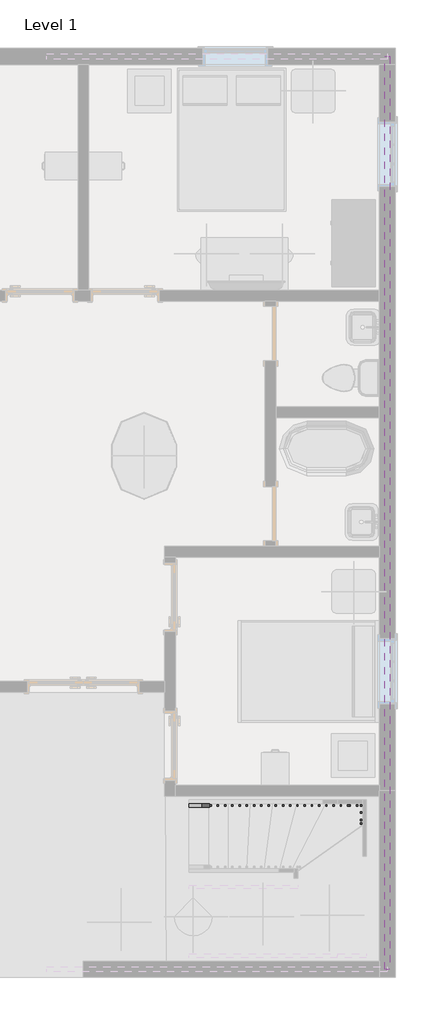
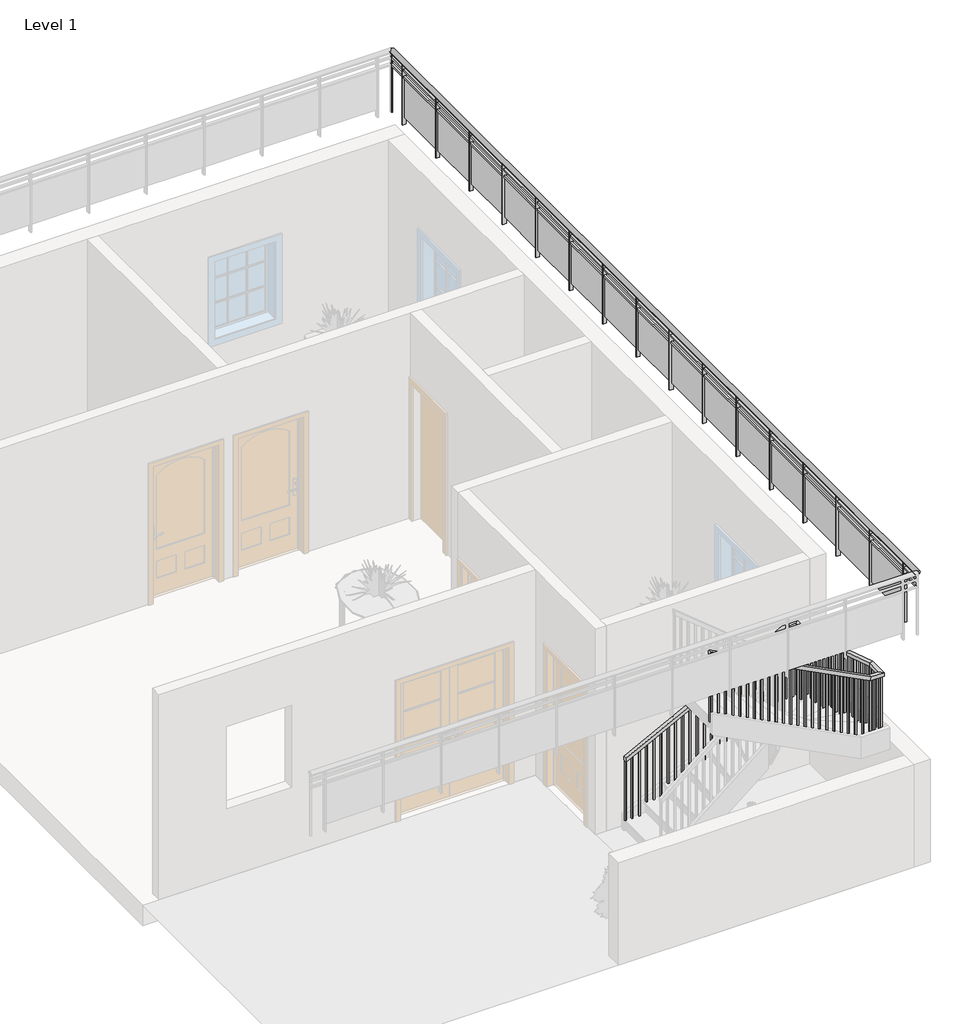
# One storey, part 3 of 4: 2 railings.
"""IFC4 building model written with IfcOpenShell, lengths in millimetres."""

from ifc_helpers import new_model, si_unit, point, frame, origin, place, context, project, spatial, polyline, ellipse_curve, trimmed, outline, extrude, faceted_brep, element, save
from ifc_brep_helpers import plane_surface, extruded_surface, advanced_brep

model = new_model("IFC4")

# Units and contexts
model_context = context("Model", 3, world=origin())
ifc_project = project(units=[si_unit("LENGTHUNIT", "METRE", prefix="MILLI")], contexts=[model_context])

# Site, building, storey
site = spatial("IfcSite", under=ifc_project)
building = spatial("IfcBuilding", under=site)
storey = spatial("IfcBuildingStorey", under=building, Name="Level 1", Elevation=0.0)

# Railings
placement = place(None, origin())
element("IfcRailing", 1, ObjectType="Glass Panel - Bottom Fill", at=placement, inside=storey, context=model_context, shape_type="SolidModel", body=[
    advanced_brep(
    [(-4161.4505662, 13087.2645941, 4267.2), (-4237.6505662, 13087.2645941, 4267.2), (-4161.4505662, 285.6645941, 4267.2), (-4237.6505662, 285.6645941, 4267.2)],
    [
        (0, 1, ellipse_curve(frame((-4199.5505662, 13087.2645941, 4267.2), z_axis=(0.0, 1.0, 0.0), x_axis=(-1.0, 0.0, 0.0)), 38.1, 28.575)),
        (1, 0, ellipse_curve(frame((-4199.5505662, 13087.2645941, 4267.2), z_axis=(0.0, 1.0, 0.0), x_axis=(-1.0, 0.0, 0.0)), 38.1, 28.575)),
        (2, 3, ellipse_curve(frame((-4199.5505662, 285.6645941, 4267.2), z_axis=(0.0, -1.0, 0.0), x_axis=(-1.0, 0.0, 0.0)), 38.1, 28.575)),
        (3, 2, ellipse_curve(frame((-4199.5505662, 285.6645941, 4267.2), z_axis=(0.0, -1.0, 0.0), x_axis=(-1.0, 0.0, 0.0)), 38.1, 28.575)),
        (0, 2),
        (3, 1),
    ],
    [
        plane_surface(frame((-4199.5505662, 13087.2645941, 4267.2), z_axis=(0.0, 1.0, 0.0), x_axis=(0.0, 0.0, -1.0))),
        plane_surface(frame((-4199.5505662, 285.6645941, 4267.2), z_axis=(0.0, -1.0, 0.0), x_axis=(0.0, 0.0, -1.0))),
        extruded_surface(trimmed(ellipse_curve(frame((-4199.5505662, 285.6645941, 4267.2), z_axis=(0.0, 1.0, 0.0), x_axis=(-1.0, 0.0, 0.0)), 38.1, 28.575), [point((-4161.4505662, 285.6645941, 4267.2))], [point((-4237.6505662, 285.6645941, 4267.2))], True, "CARTESIAN"), (0.0, 12801.599999999999, 0.0), 12801.599999999999),
        extruded_surface(trimmed(ellipse_curve(frame((-4199.5505662, 285.6645941, 4267.2), z_axis=(0.0, 1.0, 0.0), x_axis=(-1.0, 0.0, 0.0)), 38.1, 28.575), [point((-4237.6505662, 285.6645941, 4267.2))], [point((-4161.4505662, 285.6645941, 4267.2))], True, "CARTESIAN"), (0.0, 12801.599999999999, 0.0), 12801.599999999999),
    ],
    [
        (0, [[1, 2]]),
        (1, [[3, 4]]),
        (2, [[-1, 5, -4, 6]]),
        (3, [[-2, -6, -3, -5]]),
    ],
),
    extrude(outline(polyline([(-4212.2505662, 13087.2645941), (-4186.8505662, 13087.2645941), (-4186.8505662, 285.6645941), (-4212.2505662, 285.6645941), (-4212.2505662, 13087.2645941)])), frame((0.0, 0.0, 4152.9), z_axis=(0.0, 0.0, 1.0), x_axis=(1.0, 0.0, 0.0)), (0.0, 0.0, 1.0), 25.4),
    extrude(outline(polyline([(-4212.2505662, 13087.2645941), (-4186.8505662, 13087.2645941), (-4186.8505662, 285.6645941), (-4212.2505662, 285.6645941), (-4212.2505662, 13087.2645941)])), frame((0.0, 0.0, 4051.3), z_axis=(0.0, 0.0, 1.0), x_axis=(1.0, 0.0, 0.0)), (0.0, 0.0, 1.0), 25.4),
    extrude(outline(polyline([(-4224.9505662, 596.8145941), (-4174.1505662, 596.8145941), (-4174.1505662, 584.1145941), (-4224.9505662, 584.1145941), (-4224.9505662, 596.8145941)])), frame((0.0, 0.0, 3352.8), z_axis=(0.0, 0.0, 1.0), x_axis=(1.0, 0.0, 0.0)), (0.0, 0.0, 1.0), 885.6788223),
    extrude(outline(polyline([(-4193.0154092, 1403.2645941), (-4193.0154092, 590.4645941), (-4199.3654092, 590.4645941), (-4199.3654092, 1403.2645941), (-4193.0154092, 1403.2645941)])), frame((0.0, 0.0, 3454.4), z_axis=(0.0, 0.0, 1.0), x_axis=(1.0, 0.0, 0.0)), (0.0, 0.0, 1.0), 596.9),
    extrude(outline(polyline([(-4224.9505662, 1409.6145941), (-4174.1505662, 1409.6145941), (-4174.1505662, 1396.9145941), (-4224.9505662, 1396.9145941), (-4224.9505662, 1409.6145941)])), frame((0.0, 0.0, 3352.8), z_axis=(0.0, 0.0, 1.0), x_axis=(1.0, 0.0, 0.0)), (0.0, 0.0, 1.0), 885.6788223),
    extrude(outline(polyline([(-4193.0154092, 2216.0645941), (-4193.0154092, 1403.2645941), (-4199.3654092, 1403.2645941), (-4199.3654092, 2216.0645941), (-4193.0154092, 2216.0645941)])), frame((0.0, 0.0, 3454.4), z_axis=(0.0, 0.0, 1.0), x_axis=(1.0, 0.0, 0.0)), (0.0, 0.0, 1.0), 596.9),
    extrude(outline(polyline([(-4224.9505662, 2222.4145941), (-4174.1505662, 2222.4145941), (-4174.1505662, 2209.7145941), (-4224.9505662, 2209.7145941), (-4224.9505662, 2222.4145941)])), frame((0.0, 0.0, 3352.8), z_axis=(0.0, 0.0, 1.0), x_axis=(1.0, 0.0, 0.0)), (0.0, 0.0, 1.0), 885.6788223),
    extrude(outline(polyline([(-4193.0154092, 3028.8645941), (-4193.0154092, 2216.0645941), (-4199.3654092, 2216.0645941), (-4199.3654092, 3028.8645941), (-4193.0154092, 3028.8645941)])), frame((0.0, 0.0, 3454.4), z_axis=(0.0, 0.0, 1.0), x_axis=(1.0, 0.0, 0.0)), (0.0, 0.0, 1.0), 596.9),
    extrude(outline(polyline([(-4224.9505662, 3035.2145941), (-4174.1505662, 3035.2145941), (-4174.1505662, 3022.5145941), (-4224.9505662, 3022.5145941), (-4224.9505662, 3035.2145941)])), frame((0.0, 0.0, 3352.8), z_axis=(0.0, 0.0, 1.0), x_axis=(1.0, 0.0, 0.0)), (0.0, 0.0, 1.0), 885.6788223),
    extrude(outline(polyline([(-4193.0154092, 3841.6645941), (-4193.0154092, 3028.8645941), (-4199.3654092, 3028.8645941), (-4199.3654092, 3841.6645941), (-4193.0154092, 3841.6645941)])), frame((0.0, 0.0, 3454.4), z_axis=(0.0, 0.0, 1.0), x_axis=(1.0, 0.0, 0.0)), (0.0, 0.0, 1.0), 596.9),
    extrude(outline(polyline([(-4224.9505662, 3848.0145941), (-4174.1505662, 3848.0145941), (-4174.1505662, 3835.3145941), (-4224.9505662, 3835.3145941), (-4224.9505662, 3848.0145941)])), frame((0.0, 0.0, 3352.8), z_axis=(0.0, 0.0, 1.0), x_axis=(1.0, 0.0, 0.0)), (0.0, 0.0, 1.0), 885.6788223),
    extrude(outline(polyline([(-4193.0154092, 4654.4645941), (-4193.0154092, 3841.6645941), (-4199.3654092, 3841.6645941), (-4199.3654092, 4654.4645941), (-4193.0154092, 4654.4645941)])), frame((0.0, 0.0, 3454.4), z_axis=(0.0, 0.0, 1.0), x_axis=(1.0, 0.0, 0.0)), (0.0, 0.0, 1.0), 596.9),
    extrude(outline(polyline([(-4224.9505662, 4660.8145941), (-4174.1505662, 4660.8145941), (-4174.1505662, 4648.1145941), (-4224.9505662, 4648.1145941), (-4224.9505662, 4660.8145941)])), frame((0.0, 0.0, 3352.8), z_axis=(0.0, 0.0, 1.0), x_axis=(1.0, 0.0, 0.0)), (0.0, 0.0, 1.0), 885.6788223),
    extrude(outline(polyline([(-4193.0154092, 5467.2645941), (-4193.0154092, 4654.4645941), (-4199.3654092, 4654.4645941), (-4199.3654092, 5467.2645941), (-4193.0154092, 5467.2645941)])), frame((0.0, 0.0, 3454.4), z_axis=(0.0, 0.0, 1.0), x_axis=(1.0, 0.0, 0.0)), (0.0, 0.0, 1.0), 596.9),
    extrude(outline(polyline([(-4224.9505662, 5473.6145941), (-4174.1505662, 5473.6145941), (-4174.1505662, 5460.9145941), (-4224.9505662, 5460.9145941), (-4224.9505662, 5473.6145941)])), frame((0.0, 0.0, 3352.8), z_axis=(0.0, 0.0, 1.0), x_axis=(1.0, 0.0, 0.0)), (0.0, 0.0, 1.0), 885.6788223),
    extrude(outline(polyline([(-4193.0154092, 6280.0645941), (-4193.0154092, 5467.2645941), (-4199.3654092, 5467.2645941), (-4199.3654092, 6280.0645941), (-4193.0154092, 6280.0645941)])), frame((0.0, 0.0, 3454.4), z_axis=(0.0, 0.0, 1.0), x_axis=(1.0, 0.0, 0.0)), (0.0, 0.0, 1.0), 596.9),
    extrude(outline(polyline([(-4224.9505662, 6286.4145941), (-4174.1505662, 6286.4145941), (-4174.1505662, 6273.7145941), (-4224.9505662, 6273.7145941), (-4224.9505662, 6286.4145941)])), frame((0.0, 0.0, 3352.8), z_axis=(0.0, 0.0, 1.0), x_axis=(1.0, 0.0, 0.0)), (0.0, 0.0, 1.0), 885.6788223),
    extrude(outline(polyline([(-4193.0154092, 7092.8645941), (-4193.0154092, 6280.0645941), (-4199.3654092, 6280.0645941), (-4199.3654092, 7092.8645941), (-4193.0154092, 7092.8645941)])), frame((0.0, 0.0, 3454.4), z_axis=(0.0, 0.0, 1.0), x_axis=(1.0, 0.0, 0.0)), (0.0, 0.0, 1.0), 596.9),
    extrude(outline(polyline([(-4224.9505662, 7099.2145941), (-4174.1505662, 7099.2145941), (-4174.1505662, 7086.5145941), (-4224.9505662, 7086.5145941), (-4224.9505662, 7099.2145941)])), frame((0.0, 0.0, 3352.8), z_axis=(0.0, 0.0, 1.0), x_axis=(1.0, 0.0, 0.0)), (0.0, 0.0, 1.0), 885.6788223),
    extrude(outline(polyline([(-4193.0154092, 7905.6645941), (-4193.0154092, 7092.8645941), (-4199.3654092, 7092.8645941), (-4199.3654092, 7905.6645941), (-4193.0154092, 7905.6645941)])), frame((0.0, 0.0, 3454.4), z_axis=(0.0, 0.0, 1.0), x_axis=(1.0, 0.0, 0.0)), (0.0, 0.0, 1.0), 596.9),
    extrude(outline(polyline([(-4224.9505662, 7912.0145941), (-4174.1505662, 7912.0145941), (-4174.1505662, 7899.3145941), (-4224.9505662, 7899.3145941), (-4224.9505662, 7912.0145941)])), frame((0.0, 0.0, 3352.8), z_axis=(0.0, 0.0, 1.0), x_axis=(1.0, 0.0, 0.0)), (0.0, 0.0, 1.0), 885.6788223),
    extrude(outline(polyline([(-4193.0154092, 8718.4645941), (-4193.0154092, 7905.6645941), (-4199.3654092, 7905.6645941), (-4199.3654092, 8718.4645941), (-4193.0154092, 8718.4645941)])), frame((0.0, 0.0, 3454.4), z_axis=(0.0, 0.0, 1.0), x_axis=(1.0, 0.0, 0.0)), (0.0, 0.0, 1.0), 596.9),
    extrude(outline(polyline([(-4224.9505662, 8724.8145941), (-4174.1505662, 8724.8145941), (-4174.1505662, 8712.1145941), (-4224.9505662, 8712.1145941), (-4224.9505662, 8724.8145941)])), frame((0.0, 0.0, 3352.8), z_axis=(0.0, 0.0, 1.0), x_axis=(1.0, 0.0, 0.0)), (0.0, 0.0, 1.0), 885.6788223),
    extrude(outline(polyline([(-4193.0154092, 9531.2645941), (-4193.0154092, 8718.4645941), (-4199.3654092, 8718.4645941), (-4199.3654092, 9531.2645941), (-4193.0154092, 9531.2645941)])), frame((0.0, 0.0, 3454.4), z_axis=(0.0, 0.0, 1.0), x_axis=(1.0, 0.0, 0.0)), (0.0, 0.0, 1.0), 596.9),
    extrude(outline(polyline([(-4224.9505662, 9537.6145941), (-4174.1505662, 9537.6145941), (-4174.1505662, 9524.9145941), (-4224.9505662, 9524.9145941), (-4224.9505662, 9537.6145941)])), frame((0.0, 0.0, 3352.8), z_axis=(0.0, 0.0, 1.0), x_axis=(1.0, 0.0, 0.0)), (0.0, 0.0, 1.0), 885.6788223),
    extrude(outline(polyline([(-4193.0154092, 10344.0645941), (-4193.0154092, 9531.2645941), (-4199.3654092, 9531.2645941), (-4199.3654092, 10344.0645941), (-4193.0154092, 10344.0645941)])), frame((0.0, 0.0, 3454.4), z_axis=(0.0, 0.0, 1.0), x_axis=(1.0, 0.0, 0.0)), (0.0, 0.0, 1.0), 596.9),
    extrude(outline(polyline([(-4224.9505662, 10350.4145941), (-4174.1505662, 10350.4145941), (-4174.1505662, 10337.7145941), (-4224.9505662, 10337.7145941), (-4224.9505662, 10350.4145941)])), frame((0.0, 0.0, 3352.8), z_axis=(0.0, 0.0, 1.0), x_axis=(1.0, 0.0, 0.0)), (0.0, 0.0, 1.0), 885.6788223),
    extrude(outline(polyline([(-4193.0154092, 11156.8645941), (-4193.0154092, 10344.0645941), (-4199.3654092, 10344.0645941), (-4199.3654092, 11156.8645941), (-4193.0154092, 11156.8645941)])), frame((0.0, 0.0, 3454.4), z_axis=(0.0, 0.0, 1.0), x_axis=(1.0, 0.0, 0.0)), (0.0, 0.0, 1.0), 596.9),
    extrude(outline(polyline([(-4224.9505662, 11163.2145941), (-4174.1505662, 11163.2145941), (-4174.1505662, 11150.5145941), (-4224.9505662, 11150.5145941), (-4224.9505662, 11163.2145941)])), frame((0.0, 0.0, 3352.8), z_axis=(0.0, 0.0, 1.0), x_axis=(1.0, 0.0, 0.0)), (0.0, 0.0, 1.0), 885.6788223),
    extrude(outline(polyline([(-4193.0154092, 11969.6645941), (-4193.0154092, 11156.8645941), (-4199.3654092, 11156.8645941), (-4199.3654092, 11969.6645941), (-4193.0154092, 11969.6645941)])), frame((0.0, 0.0, 3454.4), z_axis=(0.0, 0.0, 1.0), x_axis=(1.0, 0.0, 0.0)), (0.0, 0.0, 1.0), 596.9),
    extrude(outline(polyline([(-4224.9505662, 11976.0145941), (-4174.1505662, 11976.0145941), (-4174.1505662, 11963.3145941), (-4224.9505662, 11963.3145941), (-4224.9505662, 11976.0145941)])), frame((0.0, 0.0, 3352.8), z_axis=(0.0, 0.0, 1.0), x_axis=(1.0, 0.0, 0.0)), (0.0, 0.0, 1.0), 885.6788223),
    extrude(outline(polyline([(-4193.0154092, 12782.4645941), (-4193.0154092, 11969.6645941), (-4199.3654092, 11969.6645941), (-4199.3654092, 12782.4645941), (-4193.0154092, 12782.4645941)])), frame((0.0, 0.0, 3454.4), z_axis=(0.0, 0.0, 1.0), x_axis=(1.0, 0.0, 0.0)), (0.0, 0.0, 1.0), 596.9),
    extrude(outline(polyline([(-4224.9505662, 12788.8145941), (-4174.1505662, 12788.8145941), (-4174.1505662, 12776.1145941), (-4224.9505662, 12776.1145941), (-4224.9505662, 12788.8145941)])), frame((0.0, 0.0, 3352.8), z_axis=(0.0, 0.0, 1.0), x_axis=(1.0, 0.0, 0.0)), (0.0, 0.0, 1.0), 885.6788223),
    extrude(outline(polyline([(-4209.0755662, 298.3645941), (-4190.0255662, 298.3645941), (-4190.0255662, 279.3145941), (-4209.0755662, 279.3145941), (-4209.0755662, 298.3645941)])), frame((0.0, 0.0, 3352.8), z_axis=(0.0, 0.0, 1.0), x_axis=(1.0, 0.0, 0.0)), (0.0, 0.0, 1.0), 885.6788223),
    extrude(outline(polyline([(-4209.0755662, 13093.6145941), (-4190.0255662, 13093.6145941), (-4190.0255662, 13074.5645941), (-4209.0755662, 13074.5645941), (-4209.0755662, 13093.6145941)])), frame((0.0, 0.0, 3352.8), z_axis=(0.0, 0.0, 1.0), x_axis=(1.0, 0.0, 0.0)), (0.0, 0.0, 1.0), 885.6788223),
])
element("IfcRailing", 2, ObjectType="Handrail - Rectangular", at=placement, inside=storey, context=model_context, shape_type="SolidModel", body=[
    faceted_brep([(-6984.582258, 2609.7645941, 1109.0771751), (-6984.582258, 2609.7645941, 1051.9280057), (-6984.582258, 2558.9645941, 1051.9280057), (-6984.582258, 2558.9645941, 1109.0771751), (-4724.6004015, 2609.7645941, 2273.7644996), (-4712.2803503, 2609.7645941, 2222.9644996), (-4712.2803503, 2558.9645941, 2222.9644996), (-4724.6004015, 2558.9645941, 2273.7644996), (-4542.4505662, 2609.7645941, 2273.7644996), (-4542.4505662, 2609.7645941, 2222.9644996), (-4593.2505662, 2558.9645941, 2222.9644996), (-4593.2505662, 2558.9645941, 2273.7644996), (-4542.4505662, 2332.6106415, 2273.7644996), (-4542.4505662, 2324.6600654, 2222.9644996), (-4593.2505662, 2324.6600654, 2222.9644996), (-4593.2505662, 2332.6106415, 2273.7644996), (-4542.4505662, 778.7185468, 2772.3688337), (-4542.4505662, 770.7679706, 2721.5688337), (-4593.2505662, 770.7679706, 2721.5688337), (-4593.2505662, 778.7185468, 2772.3688337), (-4542.4505662, 501.5645941, 2772.3688337), (-4542.4505662, 501.5645941, 2721.5688337), (-4593.2505662, 552.3645941, 2721.5688337), (-4593.2505662, 552.3645941, 2772.3688337), (-4724.6004016, 501.5645941, 2772.3688337), (-4736.9204528, 501.5645941, 2721.5688337), (-4736.9204528, 552.3645941, 2721.5688337), (-4724.6004016, 552.3645941, 2772.3688337), (-6984.582258, 501.5645941, 3937.0561582), (-6984.582258, 552.3645941, 3937.0561582), (-6984.582258, 552.3645941, 3879.9069889), (-6984.582258, 501.5645941, 3879.9069889)], [[[0, 1, 2, 3]], [[1, 0, 4, 5]], [[2, 1, 5, 6]], [[3, 2, 6, 7]], [[0, 3, 7, 4]], [[5, 4, 8, 9]], [[6, 5, 9, 10]], [[7, 6, 10, 11]], [[4, 7, 11, 8]], [[9, 8, 12, 13]], [[10, 9, 13, 14]], [[11, 10, 14, 15]], [[8, 11, 15, 12]], [[13, 12, 16, 17]], [[14, 13, 17, 18]], [[15, 14, 18, 19]], [[12, 15, 19, 16]], [[17, 16, 20, 21]], [[18, 17, 21, 22]], [[19, 18, 22, 23]], [[16, 19, 23, 20]], [[21, 20, 24, 25]], [[22, 21, 25, 26]], [[23, 22, 26, 27]], [[20, 23, 27, 24]], [[28, 29, 30, 31]], [[25, 24, 28, 31]], [[26, 25, 31, 30]], [[27, 26, 30, 29]], [[24, 27, 29, 28]]]),
    extrude(outline(polyline([(3872.0443296, -6969.3254016), (2878.6666667, -6969.3254016), (2878.6666667, -6950.2754016), (3862.2268642, -6950.2754016), (3872.0443296, -6969.3254016)])), frame((0.0, 517.4395941, 0.0), z_axis=(0.0, 1.0, 0.0), x_axis=(0.0, 0.0, 1.0)), (0.0, 0.0, 1.0), 19.05),
    extrude(outline(polyline([(3819.6845145, -6867.7254016), (2878.6666667, -6867.7254016), (2878.6666667, -6848.6754016), (3809.8670491, -6848.6754016), (3819.6845145, -6867.7254016)])), frame((0.0, 517.4395941, 0.0), z_axis=(0.0, 1.0, 0.0), x_axis=(0.0, 0.0, 1.0)), (0.0, 0.0, 1.0), 19.05),
    extrude(outline(polyline([(3767.3246993, -6766.1254016), (2878.6666667, -6766.1254016), (2878.6666667, -6747.0754016), (3757.507234, -6747.0754016), (3767.3246993, -6766.1254016)])), frame((0.0, 517.4395941, 0.0), z_axis=(0.0, 1.0, 0.0), x_axis=(0.0, 0.0, 1.0)), (0.0, 0.0, 1.0), 19.05),
    extrude(outline(polyline([(3714.9648842, -6664.5254016), (2709.3333333, -6664.5254016), (2709.3333333, -6645.4754016), (3705.1474189, -6645.4754016), (3714.9648842, -6664.5254016)])), frame((0.0, 517.4395941, 0.0), z_axis=(0.0, 1.0, 0.0), x_axis=(0.0, 0.0, 1.0)), (0.0, 0.0, 1.0), 19.05),
    extrude(outline(polyline([(3662.6050691, -6562.9254016), (2709.3333333, -6562.9254016), (2709.3333333, -6543.8754016), (3652.7876038, -6543.8754016), (3662.6050691, -6562.9254016)])), frame((0.0, 517.4395941, 0.0), z_axis=(0.0, 1.0, 0.0), x_axis=(0.0, 0.0, 1.0)), (0.0, 0.0, 1.0), 19.05),
    extrude(outline(polyline([(3610.245254, -6461.3254016), (2709.3333333, -6461.3254016), (2709.3333333, -6442.2754016), (3600.4277887, -6442.2754016), (3610.245254, -6461.3254016)])), frame((0.0, 517.4395941, 0.0), z_axis=(0.0, 1.0, 0.0), x_axis=(0.0, 0.0, 1.0)), (0.0, 0.0, 1.0), 19.05),
    extrude(outline(polyline([(3557.8854389, -6359.7254016), (2540.0, -6359.7254016), (2540.0, -6340.6754016), (3548.0679735, -6340.6754016), (3557.8854389, -6359.7254016)])), frame((0.0, 517.4395941, 0.0), z_axis=(0.0, 1.0, 0.0), x_axis=(0.0, 0.0, 1.0)), (0.0, 0.0, 1.0), 19.05),
    extrude(outline(polyline([(3505.5256238, -6258.1254016), (2540.0, -6258.1254016), (2540.0, -6239.0754016), (3495.7081584, -6239.0754016), (3505.5256238, -6258.1254016)])), frame((0.0, 517.4395941, 0.0), z_axis=(0.0, 1.0, 0.0), x_axis=(0.0, 0.0, 1.0)), (0.0, 0.0, 1.0), 19.05),
    extrude(outline(polyline([(3453.1658086, -6156.5254016), (2540.0, -6156.5254016), (2540.0, -6137.4754016), (3443.3483433, -6137.4754016), (3453.1658086, -6156.5254016)])), frame((0.0, 517.4395941, 0.0), z_axis=(0.0, 1.0, 0.0), x_axis=(0.0, 0.0, 1.0)), (0.0, 0.0, 1.0), 19.05),
    extrude(outline(polyline([(3400.8059935, -6054.9254016), (2370.6666667, -6054.9254016), (2370.6666667, -6035.8754016), (3390.9885282, -6035.8754016), (3400.8059935, -6054.9254016)])), frame((0.0, 517.4395941, 0.0), z_axis=(0.0, 1.0, 0.0), x_axis=(0.0, 0.0, 1.0)), (0.0, 0.0, 1.0), 19.05),
    extrude(outline(polyline([(3348.4461784, -5953.3254016), (2370.6666667, -5953.3254016), (2370.6666667, -5934.2754016), (3338.6287131, -5934.2754016), (3348.4461784, -5953.3254016)])), frame((0.0, 517.4395941, 0.0), z_axis=(0.0, 1.0, 0.0), x_axis=(0.0, 0.0, 1.0)), (0.0, 0.0, 1.0), 19.05),
    extrude(outline(polyline([(3296.0863633, -5851.7254016), (2370.6666667, -5851.7254016), (2370.6666667, -5832.6754016), (3286.268898, -5832.6754016), (3296.0863633, -5851.7254016)])), frame((0.0, 517.4395941, 0.0), z_axis=(0.0, 1.0, 0.0), x_axis=(0.0, 0.0, 1.0)), (0.0, 0.0, 1.0), 19.05),
    extrude(outline(polyline([(3243.7265482, -5750.1254016), (2201.3333333, -5750.1254016), (2201.3333333, -5731.0754016), (3233.9090828, -5731.0754016), (3243.7265482, -5750.1254016)])), frame((0.0, 517.4395941, 0.0), z_axis=(0.0, 1.0, 0.0), x_axis=(0.0, 0.0, 1.0)), (0.0, 0.0, 1.0), 19.05),
    extrude(outline(polyline([(3191.3667331, -5648.5254016), (2201.3333333, -5648.5254016), (2201.3333333, -5629.4754016), (3181.5492677, -5629.4754016), (3191.3667331, -5648.5254016)])), frame((0.0, 517.4395941, 0.0), z_axis=(0.0, 1.0, 0.0), x_axis=(0.0, 0.0, 1.0)), (0.0, 0.0, 1.0), 19.05),
    extrude(outline(polyline([(3139.0069179, -5546.9254016), (2201.3333333, -5546.9254016), (2201.3333333, -5527.8754016), (3129.1894526, -5527.8754016), (3139.0069179, -5546.9254016)])), frame((0.0, 517.4395941, 0.0), z_axis=(0.0, 1.0, 0.0), x_axis=(0.0, 0.0, 1.0)), (0.0, 0.0, 1.0), 19.05),
    extrude(outline(polyline([(3086.6471028, -5445.3254016), (2032.0, -5445.3254016), (2032.0, -5426.2754016), (3076.8296375, -5426.2754016), (3086.6471028, -5445.3254016)])), frame((0.0, 517.4395941, 0.0), z_axis=(0.0, 1.0, 0.0), x_axis=(0.0, 0.0, 1.0)), (0.0, 0.0, 1.0), 19.05),
    extrude(outline(polyline([(3034.2872877, -5343.7254016), (2032.0, -5343.7254016), (2032.0, -5324.6754016), (3024.4698224, -5324.6754016), (3034.2872877, -5343.7254016)])), frame((0.0, 517.4395941, 0.0), z_axis=(0.0, 1.0, 0.0), x_axis=(0.0, 0.0, 1.0)), (0.0, 0.0, 1.0), 19.05),
    extrude(outline(polyline([(2981.9274726, -5242.1254016), (2032.0, -5242.1254016), (2032.0, -5223.0754016), (2972.1100073, -5223.0754016), (2981.9274726, -5242.1254016)])), frame((0.0, 517.4395941, 0.0), z_axis=(0.0, 1.0, 0.0), x_axis=(0.0, 0.0, 1.0)), (0.0, 0.0, 1.0), 19.05),
    extrude(outline(polyline([(2929.5676575, -5140.5254016), (2032.0, -5140.5254016), (2032.0, -5121.4754016), (2919.7501921, -5121.4754016), (2929.5676575, -5140.5254016)])), frame((0.0, 517.4395941, 0.0), z_axis=(0.0, 1.0, 0.0), x_axis=(0.0, 0.0, 1.0)), (0.0, 0.0, 1.0), 19.05),
    extrude(outline(polyline([(2877.2078424, -5038.9254016), (1862.6666667, -5038.9254016), (1862.6666667, -5019.8754016), (2867.390377, -5019.8754016), (2877.2078424, -5038.9254016)])), frame((0.0, 517.4395941, 0.0), z_axis=(0.0, 1.0, 0.0), x_axis=(0.0, 0.0, 1.0)), (0.0, 0.0, 1.0), 19.05),
    extrude(outline(polyline([(2824.8480272, -4937.3254016), (1862.6666667, -4937.3254016), (1862.6666667, -4918.2754016), (2815.0305619, -4918.2754016), (2824.8480272, -4937.3254016)])), frame((0.0, 517.4395941, 0.0), z_axis=(0.0, 1.0, 0.0), x_axis=(0.0, 0.0, 1.0)), (0.0, 0.0, 1.0), 19.05),
    extrude(outline(polyline([(2772.4882121, -4835.7254016), (1862.6666667, -4835.7254016), (1862.6666667, -4816.6754016), (2762.6707468, -4816.6754016), (2772.4882121, -4835.7254016)])), frame((0.0, 517.4395941, 0.0), z_axis=(0.0, 1.0, 0.0), x_axis=(0.0, 0.0, 1.0)), (0.0, 0.0, 1.0), 19.05),
    extrude(outline(polyline([(-4659.9255662, 517.4395941), (-4678.9755662, 517.4395941), (-4678.9755662, 536.4895941), (-4659.9255662, 536.4895941), (-4659.9255662, 517.4395941)])), frame((0.0, 0.0, 1862.6666667), z_axis=(0.0, 0.0, 1.0), x_axis=(1.0, 0.0, 0.0)), (0.0, 0.0, 1.0), 858.902167),
    extrude(outline(polyline([(-4558.3255662, 585.0435468), (-4558.3255662, 565.9935468), (-4577.3755662, 565.9935468), (-4577.3755662, 585.0435468), (-4558.3255662, 585.0435468)])), frame((0.0, 0.0, 1862.6666667), z_axis=(0.0, 0.0, 1.0), x_axis=(1.0, 0.0, 0.0)), (0.0, 0.0, 1.0), 858.902167),
    extrude(outline(polyline([(-4558.3255662, 686.6435468), (-4558.3255662, 667.5935468), (-4577.3755662, 667.5935468), (-4577.3755662, 686.6435468), (-4558.3255662, 686.6435468)])), frame((0.0, 0.0, 1862.6666667), z_axis=(0.0, 0.0, 1.0), x_axis=(1.0, 0.0, 0.0)), (0.0, 0.0, 1.0), 858.902167),
    extrude(outline(polyline([(818.1356415, 2706.3697564), (818.1356415, 1693.3333333), (799.0856415, 1693.3333333), (799.0856415, 2712.4824155), (818.1356415, 2706.3697564)])), frame((-4577.3755662, 0.0, 0.0), z_axis=(1.0, 0.0, 0.0), x_axis=(0.0, 1.0, 0.0)), (0.0, 0.0, 1.0), 19.05),
    extrude(outline(polyline([(919.7356415, 2673.7689082), (919.7356415, 1693.3333333), (900.6856415, 1693.3333333), (900.6856415, 2679.8815673), (919.7356415, 2673.7689082)])), frame((-4577.3755662, 0.0, 0.0), z_axis=(1.0, 0.0, 0.0), x_axis=(0.0, 1.0, 0.0)), (0.0, 0.0, 1.0), 19.05),
    extrude(outline(polyline([(1021.3356415, 2641.16806), (1021.3356415, 1693.3333333), (1002.2856415, 1693.3333333), (1002.2856415, 2647.280719), (1021.3356415, 2641.16806)])), frame((-4577.3755662, 0.0, 0.0), z_axis=(1.0, 0.0, 0.0), x_axis=(0.0, 1.0, 0.0)), (0.0, 0.0, 1.0), 19.05),
    extrude(outline(polyline([(1122.9356415, 2608.5672118), (1122.9356415, 1693.3333333), (1103.8856415, 1693.3333333), (1103.8856415, 2614.6798708), (1122.9356415, 2608.5672118)])), frame((-4577.3755662, 0.0, 0.0), z_axis=(1.0, 0.0, 0.0), x_axis=(0.0, 1.0, 0.0)), (0.0, 0.0, 1.0), 19.05),
    extrude(outline(polyline([(1224.5356415, 2575.9663635), (1224.5356415, 1693.3333333), (1205.4856415, 1693.3333333), (1205.4856415, 2582.0790226), (1224.5356415, 2575.9663635)])), frame((-4577.3755662, 0.0, 0.0), z_axis=(1.0, 0.0, 0.0), x_axis=(0.0, 1.0, 0.0)), (0.0, 0.0, 1.0), 19.05),
    extrude(outline(polyline([(1326.1356415, 2543.3655153), (1326.1356415, 1693.3333333), (1307.0856415, 1693.3333333), (1307.0856415, 2549.4781744), (1326.1356415, 2543.3655153)])), frame((-4577.3755662, 0.0, 0.0), z_axis=(1.0, 0.0, 0.0), x_axis=(0.0, 1.0, 0.0)), (0.0, 0.0, 1.0), 19.05),
    extrude(outline(polyline([(1427.7356415, 2510.7646671), (1427.7356415, 1524.0), (1408.6856415, 1524.0), (1408.6856415, 2516.8773261), (1427.7356415, 2510.7646671)])), frame((-4577.3755662, 0.0, 0.0), z_axis=(1.0, 0.0, 0.0), x_axis=(0.0, 1.0, 0.0)), (0.0, 0.0, 1.0), 19.05),
    extrude(outline(polyline([(1529.3356415, 2478.1638189), (1529.3356415, 1524.0), (1510.2856415, 1524.0), (1510.2856415, 2484.2764779), (1529.3356415, 2478.1638189)])), frame((-4577.3755662, 0.0, 0.0), z_axis=(1.0, 0.0, 0.0), x_axis=(0.0, 1.0, 0.0)), (0.0, 0.0, 1.0), 19.05),
    extrude(outline(polyline([(1630.9356415, 2445.5629706), (1630.9356415, 1524.0), (1611.8856415, 1524.0), (1611.8856415, 2451.6756297), (1630.9356415, 2445.5629706)])), frame((-4577.3755662, 0.0, 0.0), z_axis=(1.0, 0.0, 0.0), x_axis=(0.0, 1.0, 0.0)), (0.0, 0.0, 1.0), 19.05),
    extrude(outline(polyline([(1732.5356415, 2412.9621224), (1732.5356415, 1524.0), (1713.4856415, 1524.0), (1713.4856415, 2419.0747814), (1732.5356415, 2412.9621224)])), frame((-4577.3755662, 0.0, 0.0), z_axis=(1.0, 0.0, 0.0), x_axis=(0.0, 1.0, 0.0)), (0.0, 0.0, 1.0), 19.05),
    extrude(outline(polyline([(1834.1356415, 2380.3612742), (1834.1356415, 1354.6666667), (1815.0856415, 1354.6666667), (1815.0856415, 2386.4739332), (1834.1356415, 2380.3612742)])), frame((-4577.3755662, 0.0, 0.0), z_axis=(1.0, 0.0, 0.0), x_axis=(0.0, 1.0, 0.0)), (0.0, 0.0, 1.0), 19.05),
    extrude(outline(polyline([(1935.7356415, 2347.7604259), (1935.7356415, 1354.6666667), (1916.6856415, 1354.6666667), (1916.6856415, 2353.873085), (1935.7356415, 2347.7604259)])), frame((-4577.3755662, 0.0, 0.0), z_axis=(1.0, 0.0, 0.0), x_axis=(0.0, 1.0, 0.0)), (0.0, 0.0, 1.0), 19.05),
    extrude(outline(polyline([(2037.3356415, 2315.1595777), (2037.3356415, 1354.6666667), (2018.2856415, 1354.6666667), (2018.2856415, 2321.2722368), (2037.3356415, 2315.1595777)])), frame((-4577.3755662, 0.0, 0.0), z_axis=(1.0, 0.0, 0.0), x_axis=(0.0, 1.0, 0.0)), (0.0, 0.0, 1.0), 19.05),
    extrude(outline(polyline([(2138.9356415, 2282.5587295), (2138.9356415, 1354.6666667), (2119.8856415, 1354.6666667), (2119.8856415, 2288.6713885), (2138.9356415, 2282.5587295)])), frame((-4577.3755662, 0.0, 0.0), z_axis=(1.0, 0.0, 0.0), x_axis=(0.0, 1.0, 0.0)), (0.0, 0.0, 1.0), 19.05),
    extrude(outline(polyline([(2240.5356415, 2249.9578813), (2240.5356415, 1354.6666667), (2221.4856415, 1354.6666667), (2221.4856415, 2256.0705403), (2240.5356415, 2249.9578813)])), frame((-4577.3755662, 0.0, 0.0), z_axis=(1.0, 0.0, 0.0), x_axis=(0.0, 1.0, 0.0)), (0.0, 0.0, 1.0), 19.05),
    extrude(outline(polyline([(-4558.3255662, 2390.6895941), (-4558.3255662, 2371.6395941), (-4577.3755662, 2371.6395941), (-4577.3755662, 2390.6895941), (-4558.3255662, 2390.6895941)])), frame((0.0, 0.0, 1185.3333333), z_axis=(0.0, 0.0, 1.0), x_axis=(1.0, 0.0, 0.0)), (0.0, 0.0, 1.0), 1037.6311663),
    extrude(outline(polyline([(-4558.3255662, 2492.2895941), (-4558.3255662, 2473.2395941), (-4577.3755662, 2473.2395941), (-4577.3755662, 2492.2895941), (-4558.3255662, 2492.2895941)])), frame((0.0, 0.0, 1185.3333333), z_axis=(0.0, 0.0, 1.0), x_axis=(1.0, 0.0, 0.0)), (0.0, 0.0, 1.0), 1037.6311663),
    extrude(outline(polyline([(-4632.5254015, 2593.8895941), (-4613.4754015, 2593.8895941), (-4613.4754015, 2574.8395941), (-4632.5254015, 2574.8395941), (-4632.5254015, 2593.8895941)])), frame((0.0, 0.0, 1185.3333333), z_axis=(0.0, 0.0, 1.0), x_axis=(1.0, 0.0, 0.0)), (0.0, 0.0, 1.0), 1037.6311663),
    extrude(outline(polyline([(2198.9352056, -4758.907258), (1185.3333333, -4758.907258), (1185.3333333, -4739.857258), (2208.752671, -4739.857258), (2198.9352056, -4758.907258)])), frame((0.0, 2574.8395941, 0.0), z_axis=(0.0, 1.0, 0.0), x_axis=(0.0, 0.0, 1.0)), (0.0, 0.0, 1.0), 19.05),
    extrude(outline(polyline([(2146.5753905, -4860.507258), (1185.3333333, -4860.507258), (1185.3333333, -4841.457258), (2156.3928558, -4841.457258), (2146.5753905, -4860.507258)])), frame((0.0, 2574.8395941, 0.0), z_axis=(0.0, 1.0, 0.0), x_axis=(0.0, 0.0, 1.0)), (0.0, 0.0, 1.0), 19.05),
    extrude(outline(polyline([(2094.2155754, -4962.107258), (1185.3333333, -4962.107258), (1185.3333333, -4943.057258), (2104.0330407, -4943.057258), (2094.2155754, -4962.107258)])), frame((0.0, 2574.8395941, 0.0), z_axis=(0.0, 1.0, 0.0), x_axis=(0.0, 0.0, 1.0)), (0.0, 0.0, 1.0), 19.05),
    extrude(outline(polyline([(2041.8557603, -5063.707258), (1185.3333333, -5063.707258), (1185.3333333, -5044.657258), (2051.6732256, -5044.657258), (2041.8557603, -5063.707258)])), frame((0.0, 2574.8395941, 0.0), z_axis=(0.0, 1.0, 0.0), x_axis=(0.0, 0.0, 1.0)), (0.0, 0.0, 1.0), 19.05),
    extrude(outline(polyline([(1989.4959452, -5165.307258), (1016.0, -5165.307258), (1016.0, -5146.257258), (1999.3134105, -5146.257258), (1989.4959452, -5165.307258)])), frame((0.0, 2574.8395941, 0.0), z_axis=(0.0, 1.0, 0.0), x_axis=(0.0, 0.0, 1.0)), (0.0, 0.0, 1.0), 19.05),
    extrude(outline(polyline([(1937.13613, -5266.907258), (1016.0, -5266.907258), (1016.0, -5247.857258), (1946.9535954, -5247.857258), (1937.13613, -5266.907258)])), frame((0.0, 2574.8395941, 0.0), z_axis=(0.0, 1.0, 0.0), x_axis=(0.0, 0.0, 1.0)), (0.0, 0.0, 1.0), 19.05),
    extrude(outline(polyline([(1884.7763149, -5368.507258), (1016.0, -5368.507258), (1016.0, -5349.457258), (1894.5937803, -5349.457258), (1884.7763149, -5368.507258)])), frame((0.0, 2574.8395941, 0.0), z_axis=(0.0, 1.0, 0.0), x_axis=(0.0, 0.0, 1.0)), (0.0, 0.0, 1.0), 19.05),
    extrude(outline(polyline([(1832.4164998, -5470.107258), (1016.0, -5470.107258), (1016.0, -5451.057258), (1842.2339651, -5451.057258), (1832.4164998, -5470.107258)])), frame((0.0, 2574.8395941, 0.0), z_axis=(0.0, 1.0, 0.0), x_axis=(0.0, 0.0, 1.0)), (0.0, 0.0, 1.0), 19.05),
    extrude(outline(polyline([(1780.0566847, -5571.707258), (846.6666667, -5571.707258), (846.6666667, -5552.657258), (1789.87415, -5552.657258), (1780.0566847, -5571.707258)])), frame((0.0, 2574.8395941, 0.0), z_axis=(0.0, 1.0, 0.0), x_axis=(0.0, 0.0, 1.0)), (0.0, 0.0, 1.0), 19.05),
    extrude(outline(polyline([(1727.6968696, -5673.307258), (846.6666667, -5673.307258), (846.6666667, -5654.257258), (1737.5143349, -5654.257258), (1727.6968696, -5673.307258)])), frame((0.0, 2574.8395941, 0.0), z_axis=(0.0, 1.0, 0.0), x_axis=(0.0, 0.0, 1.0)), (0.0, 0.0, 1.0), 19.05),
    extrude(outline(polyline([(1675.3370545, -5774.907258), (846.6666667, -5774.907258), (846.6666667, -5755.857258), (1685.1545198, -5755.857258), (1675.3370545, -5774.907258)])), frame((0.0, 2574.8395941, 0.0), z_axis=(0.0, 1.0, 0.0), x_axis=(0.0, 0.0, 1.0)), (0.0, 0.0, 1.0), 19.05),
    extrude(outline(polyline([(1622.9772393, -5876.507258), (677.3333333, -5876.507258), (677.3333333, -5857.457258), (1632.7947047, -5857.457258), (1622.9772393, -5876.507258)])), frame((0.0, 2574.8395941, 0.0), z_axis=(0.0, 1.0, 0.0), x_axis=(0.0, 0.0, 1.0)), (0.0, 0.0, 1.0), 19.05),
    extrude(outline(polyline([(1570.6174242, -5978.107258), (677.3333333, -5978.107258), (677.3333333, -5959.057258), (1580.4348896, -5959.057258), (1570.6174242, -5978.107258)])), frame((0.0, 2574.8395941, 0.0), z_axis=(0.0, 1.0, 0.0), x_axis=(0.0, 0.0, 1.0)), (0.0, 0.0, 1.0), 19.05),
    extrude(outline(polyline([(1518.2576091, -6079.707258), (677.3333333, -6079.707258), (677.3333333, -6060.657258), (1528.0750744, -6060.657258), (1518.2576091, -6079.707258)])), frame((0.0, 2574.8395941, 0.0), z_axis=(0.0, 1.0, 0.0), x_axis=(0.0, 0.0, 1.0)), (0.0, 0.0, 1.0), 19.05),
    extrude(outline(polyline([(1465.897794, -6181.307258), (508.0, -6181.307258), (508.0, -6162.257258), (1475.7152593, -6162.257258), (1465.897794, -6181.307258)])), frame((0.0, 2574.8395941, 0.0), z_axis=(0.0, 1.0, 0.0), x_axis=(0.0, 0.0, 1.0)), (0.0, 0.0, 1.0), 19.05),
    extrude(outline(polyline([(1413.5379789, -6282.907258), (508.0, -6282.907258), (508.0, -6263.857258), (1423.3554442, -6263.857258), (1413.5379789, -6282.907258)])), frame((0.0, 2574.8395941, 0.0), z_axis=(0.0, 1.0, 0.0), x_axis=(0.0, 0.0, 1.0)), (0.0, 0.0, 1.0), 19.05),
    extrude(outline(polyline([(1361.1781638, -6384.507258), (508.0, -6384.507258), (508.0, -6365.457258), (1370.9956291, -6365.457258), (1361.1781638, -6384.507258)])), frame((0.0, 2574.8395941, 0.0), z_axis=(0.0, 1.0, 0.0), x_axis=(0.0, 0.0, 1.0)), (0.0, 0.0, 1.0), 19.05),
    extrude(outline(polyline([(1308.8183486, -6486.107258), (338.6666667, -6486.107258), (338.6666667, -6467.057258), (1318.635814, -6467.057258), (1308.8183486, -6486.107258)])), frame((0.0, 2574.8395941, 0.0), z_axis=(0.0, 1.0, 0.0), x_axis=(0.0, 0.0, 1.0)), (0.0, 0.0, 1.0), 19.05),
    extrude(outline(polyline([(1256.4585335, -6587.707258), (338.6666667, -6587.707258), (338.6666667, -6568.657258), (1266.2759989, -6568.657258), (1256.4585335, -6587.707258)])), frame((0.0, 2574.8395941, 0.0), z_axis=(0.0, 1.0, 0.0), x_axis=(0.0, 0.0, 1.0)), (0.0, 0.0, 1.0), 19.05),
    extrude(outline(polyline([(1204.0987184, -6689.307258), (338.6666667, -6689.307258), (338.6666667, -6670.257258), (1213.9161837, -6670.257258), (1204.0987184, -6689.307258)])), frame((0.0, 2574.8395941, 0.0), z_axis=(0.0, 1.0, 0.0), x_axis=(0.0, 0.0, 1.0)), (0.0, 0.0, 1.0), 19.05),
    extrude(outline(polyline([(1151.7389033, -6790.907258), (169.3333333, -6790.907258), (169.3333333, -6771.857258), (1161.5563686, -6771.857258), (1151.7389033, -6790.907258)])), frame((0.0, 2574.8395941, 0.0), z_axis=(0.0, 1.0, 0.0), x_axis=(0.0, 0.0, 1.0)), (0.0, 0.0, 1.0), 19.05),
    extrude(outline(polyline([(1099.3790882, -6892.507258), (169.3333333, -6892.507258), (169.3333333, -6873.457258), (1109.1965535, -6873.457258), (1099.3790882, -6892.507258)])), frame((0.0, 2574.8395941, 0.0), z_axis=(0.0, 1.0, 0.0), x_axis=(0.0, 0.0, 1.0)), (0.0, 0.0, 1.0), 19.05),
    extrude(outline(polyline([(-4715.0754016, 517.4395941), (-4734.1254016, 517.4395941), (-4734.1254016, 536.4895941), (-4715.0754016, 536.4895941), (-4715.0754016, 517.4395941)])), frame((0.0, 0.0, 1862.6666667), z_axis=(0.0, 0.0, 1.0), x_axis=(1.0, 0.0, 0.0)), (0.0, 0.0, 1.0), 858.902167),
    extrude(outline(polyline([(-4558.3255662, 536.4895941), (-4558.3255662, 517.4395941), (-4577.3755662, 517.4395941), (-4577.3755662, 536.4895941), (-4558.3255662, 536.4895941)])), frame((0.0, 0.0, 1862.6666667), z_axis=(0.0, 0.0, 1.0), x_axis=(1.0, 0.0, 0.0)), (0.0, 0.0, 1.0), 858.902167),
    extrude(outline(polyline([(788.2435468, 2715.9613671), (788.2435468, 1862.6666667), (769.1935468, 1862.6666667), (769.1935468, 2722.0740262), (788.2435468, 2715.9613671)])), frame((-4577.3755662, 0.0, 0.0), z_axis=(1.0, 0.0, 0.0), x_axis=(0.0, 1.0, 0.0)), (0.0, 0.0, 1.0), 19.05),
    extrude(outline(polyline([(-4558.3255662, 2342.1356415), (-4558.3255662, 2323.0856415), (-4577.3755662, 2323.0856415), (-4577.3755662, 2342.1356415), (-4558.3255662, 2342.1356415)])), frame((0.0, 0.0, 1185.3333333), z_axis=(0.0, 0.0, 1.0), x_axis=(1.0, 0.0, 0.0)), (0.0, 0.0, 1.0), 1037.6311663),
    extrude(outline(polyline([(-4577.3755662, 2593.8895941), (-4558.3255662, 2593.8895941), (-4558.3255662, 2574.8395941), (-4577.3755662, 2574.8395941), (-4577.3755662, 2593.8895941)])), frame((0.0, 0.0, 1185.3333333), z_axis=(0.0, 0.0, 1.0), x_axis=(1.0, 0.0, 0.0)), (0.0, 0.0, 1.0), 1037.6311663),
    extrude(outline(polyline([(2211.7065976, -4734.1254015), (1185.3333333, -4734.1254015), (1185.3333333, -4715.0754015), (2221.5240629, -4715.0754015), (2211.7065976, -4734.1254015)])), frame((0.0, 2574.8395941, 0.0), z_axis=(0.0, 1.0, 0.0), x_axis=(0.0, 0.0, 1.0)), (0.0, 0.0, 1.0), 19.05),
    extrude(outline(polyline([(3879.9069889, -6984.582258), (2878.6666667, -6984.582258), (2878.6666667, -6965.532258), (3870.0895235, -6965.532258), (3879.9069889, -6984.582258)])), frame((0.0, 517.4395941, 0.0), z_axis=(0.0, 1.0, 0.0), x_axis=(0.0, 0.0, 1.0)), (0.0, 0.0, 1.0), 19.05),
    extrude(outline(polyline([(1051.9280057, -6984.582258), (169.3333333, -6984.582258), (169.3333333, -6965.532258), (1061.7454711, -6965.532258), (1051.9280057, -6984.582258)])), frame((0.0, 2574.8395941, 0.0), z_axis=(0.0, 1.0, 0.0), x_axis=(0.0, 0.0, 1.0)), (0.0, 0.0, 1.0), 19.05),
])

save(model, "model.ifc")

# Revit data of these elements
# Type "Glass Panel - Bottom Fill"
#   Assembly Code = "C2010400"
#   built-in parameter 1008612 = 0.0416667 (stored number, unit not read)
#   built-in parameter 1008611 = 0.0416667 (stored number, unit not read)
#   built-in parameter 1008609 = 0.333333 (stored number, unit not read)
#   built-in parameter 1008604 = 0.166667 (stored number, unit not read)
#   built-in parameter 1008603 = 0.166667 (stored number, unit not read)
#   Railing Height = 3' - 0"
#   built-in parameter 1008630 = 2
#   built-in parameter 1008610 = 2
#   built-in parameter 1008618 = Baluster - Square : 3/4"
# Type "Handrail - Rectangular"
#   Assembly Code = "C2010400"
#   built-in parameter 1008612 = 0.0416667 (stored number, unit not read)
#   built-in parameter 1008611 = 0.0416667 (stored number, unit not read)
#   built-in parameter 1008609 = 0.333333 (stored number, unit not read)
#   built-in parameter 1008604 = 0.166667 (stored number, unit not read)
#   built-in parameter 1008603 = 0.166667 (stored number, unit not read)
#   Railing Height = 3' - 0"
#   built-in parameter 1008630 = 2
#   built-in parameter 1008610 = 2
#   built-in parameter 1008618 = Baluster - Square : 3/4"
# Element 1 (IfcRailing, "Glass Panel - Bottom Fill")
#   built-in parameter 1008621 = 11 (stored number, unit not read)
#   Phase Created = New Construction
#   Materials on its faces: "Glass"
# Element 2 (IfcRailing, "Handrail - Rectangular")
#   Phase Created = New Construction
# Materials
#   "Glass": class "Glass", colour RGB 0 128 192, transparency 0.75, Description = "Soda Lime Glass", Cost = 0
